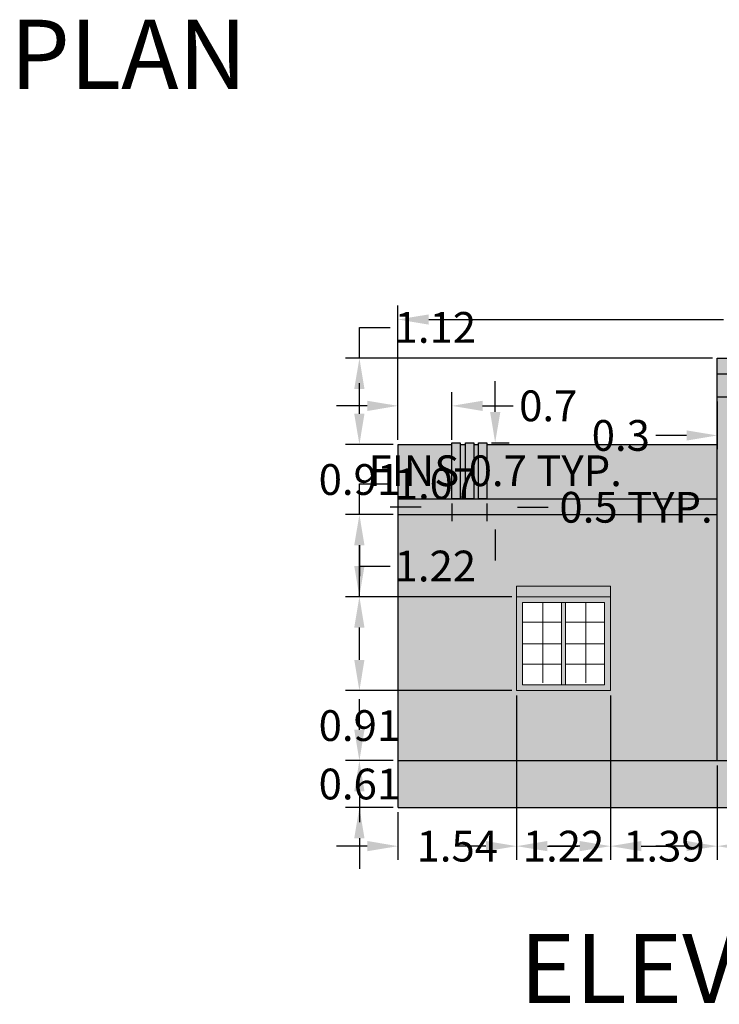
# Model space of a CAD drawing. Units: metres. Extents: x 24.2 to 58.5, y -14.5 to 15.2.
# Tile 1 of 7: x 29.8 to 38.9, y -14.5 to -1.7. Entities that reach past the tile are written whole.
import ezdxf

# ---------------------------------------------------------------- set-up
doc = ezdxf.new("R2010")
doc.units = ezdxf.units.M
doc.header["$MEASUREMENT"] = 0
for name, color, linetype, lineweight in [('A-ANNO-TITL', 1, 'Continuous', 30), ('A-ELEV', 7, 'Continuous', 25), ('A-ELEV-PATT', 61, 'Continuous', 13), ('A-GLAZ', 15, 'Continuous', 18), ('DIMENSION', 90, 'Continuous', 18)]:
    doc.layers.add(name, color=color, linetype=linetype, lineweight=lineweight)
doc.layers.add('A-ELEV-TRIM-PATT', color=251, linetype='Continuous', lineweight=13, true_color=0x636466)
doc.styles.get("Standard").update_dxf_attribs({"font": 'arial.ttf'})
doc.dimstyles.get("Standard").update_dxf_attribs({"dimtxt": 0.4, "dimasz": 0.4, "dimexe": 0.18, "dimexo": 0.0625, "dimgap": 0.09, "dimtad": 0, "dimtih": 1, "dimtoh": 1, "dimdec": 1, "dimzin": 0, "dimdsep": 46, "dimtxsty": 'Standard', "dimcen": 0.09, "dimadec": 0, "dimazin": 0, "dimtfac": 1, "dimtdec": 1, "dimtofl": 0, "dimtmove": 0, "dimatfit": 3, "dimfxl": 1, "dimtolj": 1, "dimtzin": 0, "dimarcsym": 0})

# ---------------------------------------------------------------- blocks, each defined once
blk = doc.blocks.new('PARAPET-TRIPLE-FIN')
for p, q in [((0.11, 0.707), (0.177, 0.707)), ((0.286, 0.707), (0.345, 0.707))]:
    blk.add_line(p, q)
for points in [[(0, 0.731), (0.11, 0.731), (0.11, 0), (0, 0)], [(0, 0.731), (0.11, 0.731), (0.11, 0), (0, 0)], [(0.177, 0.731), (0.286, 0.731), (0.286, 0), (0.177, 0)], [(0.345, 0.731), (0.455, 0.731), (0.455, 0), (0.345, 0)]]:
    blk.add_lwpolyline(points, close=True)
blk = doc.blocks.new('*D67')
at = {"layer": 'Defpoints', "color": 0, "transparency": 16777216}
for p in [(35.829, -7.164), (35.938, -7.164), (35.829, -7.895)]:
    blk.add_point(p, dxfattribs=at)
at = {"layer": 'DIMENSION', "color": 0, "lineweight": -2, "transparency": 16777216}
for p, q in [((35.938, -6.764), (35.938, -6.364)), ((35.891, -7.164), (36.118, -7.164)), ((35.891, -7.895), (36.118, -7.895)), ((35.938, -8.295), (35.938, -8.695))]:
    blk.add_line(p, q, dxfattribs=at)
at = {"layer": 'DIMENSION', "color": 0, "transparency": 16777216}
for points in [[(35.872, -6.764), (36.005, -6.764), (35.938, -7.164)], [(35.872, -8.295), (36.005, -8.295), (35.938, -7.895)]]:
    blk.add_solid(points, dxfattribs=at)
at = {"layer": 'DIMENSION', "color": 0, "transparency": 16777216, "insert": (35.938, -7.529), "char_height": 0.4, "attachment_point": 5}
blk.add_mtext('\\A1;FINS 0.7 TYP.', dxfattribs=at)
blk = doc.blocks.new('*D68')
at = {"layer": 'Defpoints', "color": 0, "transparency": 16777216}
for p in [(35.374, -7.895), (35.829, -7.895), (35.829, -8.004)]:
    blk.add_point(p, dxfattribs=at)
at = {"layer": 'DIMENSION', "color": 0, "lineweight": -2, "transparency": 16777216}
for p, q in [((34.974, -8.004), (34.574, -8.004)), ((35.374, -7.957), (35.374, -8.184)), ((35.829, -7.957), (35.829, -8.184)), ((36.229, -8.004), (36.629, -8.004))]:
    blk.add_line(p, q, dxfattribs=at)
at = {"layer": 'DIMENSION', "color": 0, "transparency": 16777216}
for points in [[(34.974, -7.938), (34.974, -8.071), (35.374, -8.004)], [(36.229, -7.938), (36.229, -8.071), (35.829, -8.004)]]:
    blk.add_solid(points, dxfattribs=at)
at = {"layer": 'DIMENSION', "color": 0, "transparency": 16777216, "insert": (37.77, -8.004), "char_height": 0.4, "attachment_point": 5}
blk.add_mtext('\\A1;0.5 TYP.', dxfattribs=at)
blk = doc.blocks.new('*D81')
at = {"layer": 'Defpoints', "color": 0, "transparency": 16777216}
for p in [(44.284, -5.562), (34.674, -7.188), (44.284, -7.188)]:
    blk.add_point(p, dxfattribs=at)
at = {"layer": 'DIMENSION', "color": 0, "lineweight": -2, "transparency": 16777216}
for p, q in [((34.674, -7.125), (34.674, -5.382)), ((44.284, -7.125), (44.284, -5.382)), ((35.074, -5.562), (38.908, -5.562)), ((43.884, -5.562), (40.05, -5.562))]:
    blk.add_line(p, q, dxfattribs=at)
at = {"layer": 'DIMENSION', "color": 0, "transparency": 16777216}
for points in [[(35.074, -5.496), (35.074, -5.629), (34.674, -5.562)], [(43.884, -5.496), (43.884, -5.629), (44.284, -5.562)]]:
    blk.add_solid(points, dxfattribs=at)
at = {"layer": 'DIMENSION', "color": 0, "transparency": 16777216, "insert": (39.479, -5.562), "char_height": 0.4, "attachment_point": 5}
blk.add_mtext('\\A1;9.61', dxfattribs=at)
blk = doc.blocks.new('*D83')
at = {"layer": 'Defpoints', "color": 0, "transparency": 16777216}
for p in [(34.172, -11.298), (34.674, -11.298), (34.674, -11.908)]:
    blk.add_point(p, dxfattribs=at)
at = {"layer": 'DIMENSION', "color": 0, "lineweight": -2, "transparency": 16777216}
for p, q in [((34.172, -10.898), (34.172, -10.498)), ((34.612, -11.298), (33.992, -11.298)), ((34.612, -11.908), (33.992, -11.908)), ((34.172, -12.308), (34.172, -12.708))]:
    blk.add_line(p, q, dxfattribs=at)
at = {"layer": 'DIMENSION', "color": 0, "transparency": 16777216}
for points in [[(34.105, -10.898), (34.238, -10.898), (34.172, -11.298)], [(34.105, -12.308), (34.238, -12.308), (34.172, -11.908)]]:
    blk.add_solid(points, dxfattribs=at)
at = {"layer": 'DIMENSION', "color": 0, "transparency": 16777216, "insert": (34.172, -11.603), "char_height": 0.4, "attachment_point": 5}
blk.add_mtext('\\A1;0.61', dxfattribs=at)
blk = doc.blocks.new('*D84')
at = {"layer": 'Defpoints', "color": 0, "transparency": 16777216}
for p in [(34.172, -10.388), (36.217, -10.388), (34.674, -11.298)]:
    blk.add_point(p, dxfattribs=at)
at = {"layer": 'DIMENSION', "color": 0, "lineweight": -2, "transparency": 16777216}
for p, q in [((34.172, -9.988), (34.172, -9.588)), ((36.154, -10.388), (33.992, -10.388)), ((34.612, -11.298), (33.992, -11.298)), ((34.172, -11.698), (34.172, -12.098))]:
    blk.add_line(p, q, dxfattribs=at)
at = {"layer": 'DIMENSION', "color": 0, "transparency": 16777216}
for points in [[(34.105, -9.988), (34.238, -9.988), (34.172, -10.388)], [(34.105, -11.698), (34.238, -11.698), (34.172, -11.298)]]:
    blk.add_solid(points, dxfattribs=at)
at = {"layer": 'DIMENSION', "color": 0, "transparency": 16777216, "insert": (34.172, -10.843), "char_height": 0.4, "attachment_point": 5}
blk.add_mtext('\\A1;0.91', dxfattribs=at)
blk = doc.blocks.new('*D85')
at = {"layer": 'Defpoints', "color": 0, "transparency": 16777216}
for p in [(34.172, -9.168), (36.217, -9.168), (36.217, -10.388)]:
    blk.add_point(p, dxfattribs=at)
at = {"layer": 'DIMENSION', "color": 0, "lineweight": -2, "transparency": 16777216}
for p, q in [((34.172, -9.168), (34.172, -8.768)), ((34.172, -8.768), (34.572, -8.768)), ((36.154, -9.168), (33.992, -9.168)), ((34.172, -9.988), (34.172, -9.568)), ((36.154, -10.388), (33.992, -10.388))]:
    blk.add_line(p, q, dxfattribs=at)
at = {"layer": 'DIMENSION', "color": 0, "transparency": 16777216}
for points in [[(34.105, -9.568), (34.238, -9.568), (34.172, -9.168)], [(34.105, -9.988), (34.238, -9.988), (34.172, -10.388)]]:
    blk.add_solid(points, dxfattribs=at)
at = {"layer": 'DIMENSION', "color": 0, "transparency": 16777216, "insert": (35.16, -8.768), "char_height": 0.4, "attachment_point": 5}
blk.add_mtext('\\A1;1.22', dxfattribs=at)
blk = doc.blocks.new('*D86')
at = {"layer": 'Defpoints', "color": 0, "transparency": 16777216}
for p in [(34.172, -8.098), (34.674, -8.098), (36.217, -9.168)]:
    blk.add_point(p, dxfattribs=at)
at = {"layer": 'DIMENSION', "color": 0, "lineweight": -2, "transparency": 16777216}
for p, q in [((34.172, -8.098), (34.172, -7.698)), ((34.172, -7.698), (34.572, -7.698)), ((34.612, -8.098), (33.992, -8.098)), ((34.172, -8.768), (34.172, -8.498)), ((36.154, -9.168), (33.992, -9.168))]:
    blk.add_line(p, q, dxfattribs=at)
at = {"layer": 'DIMENSION', "color": 0, "transparency": 16777216}
for points in [[(34.105, -8.498), (34.238, -8.498), (34.172, -8.098)], [(34.105, -8.768), (34.238, -8.768), (34.172, -9.168)]]:
    blk.add_solid(points, dxfattribs=at)
at = {"layer": 'DIMENSION', "color": 0, "transparency": 16777216, "insert": (35.162, -7.698), "char_height": 0.4, "attachment_point": 5}
blk.add_mtext('\\A1;1.07', dxfattribs=at)
blk = doc.blocks.new('*D87')
at = {"layer": 'Defpoints', "color": 0, "transparency": 16777216}
for p in [(34.172, -7.188), (34.674, -7.188), (34.674, -8.098)]:
    blk.add_point(p, dxfattribs=at)
at = {"layer": 'DIMENSION', "color": 0, "lineweight": -2, "transparency": 16777216}
for p, q in [((34.172, -6.788), (34.172, -6.388)), ((34.612, -7.188), (33.992, -7.188)), ((34.612, -8.098), (33.992, -8.098)), ((34.172, -8.498), (34.172, -8.898))]:
    blk.add_line(p, q, dxfattribs=at)
at = {"layer": 'DIMENSION', "color": 0, "transparency": 16777216}
for points in [[(34.105, -6.788), (34.238, -6.788), (34.172, -7.188)], [(34.105, -8.498), (34.238, -8.498), (34.172, -8.098)]]:
    blk.add_solid(points, dxfattribs=at)
at = {"layer": 'DIMENSION', "color": 0, "transparency": 16777216, "insert": (34.172, -7.643), "char_height": 0.4, "attachment_point": 5}
blk.add_mtext('\\A1;0.91', dxfattribs=at)
blk = doc.blocks.new('*D88')
at = {"layer": 'Defpoints', "color": 0, "transparency": 16777216}
for p in [(34.172, -6.065), (38.827, -6.065), (34.674, -7.188)]:
    blk.add_point(p, dxfattribs=at)
at = {"layer": 'DIMENSION', "color": 0, "lineweight": -2, "transparency": 16777216}
for p, q in [((34.172, -6.065), (34.172, -5.665)), ((34.172, -5.665), (34.572, -5.665)), ((38.764, -6.065), (33.992, -6.065)), ((34.172, -6.788), (34.172, -6.465)), ((34.612, -7.188), (33.992, -7.188))]:
    blk.add_line(p, q, dxfattribs=at)
at = {"layer": 'DIMENSION', "color": 0, "transparency": 16777216}
for points in [[(34.105, -6.465), (34.238, -6.465), (34.172, -6.065)], [(34.105, -6.788), (34.238, -6.788), (34.172, -7.188)]]:
    blk.add_solid(points, dxfattribs=at)
at = {"layer": 'DIMENSION', "color": 0, "transparency": 16777216, "insert": (35.16, -5.665), "char_height": 0.4, "attachment_point": 5}
blk.add_mtext('\\A1;1.12', dxfattribs=at)
blk = doc.blocks.new('*D90')
at = {"layer": 'Defpoints', "color": 0, "transparency": 16777216}
for p in [(36.217, -10.388), (34.674, -11.908), (36.217, -12.411)]:
    blk.add_point(p, dxfattribs=at)
at = {"layer": 'DIMENSION', "color": 0, "lineweight": -2, "transparency": 16777216}
for p, q in [((36.217, -10.451), (36.217, -12.591)), ((34.674, -11.971), (34.674, -12.591)), ((34.274, -12.411), (33.874, -12.411)), ((36.617, -12.411), (37.017, -12.411))]:
    blk.add_line(p, q, dxfattribs=at)
at = {"layer": 'DIMENSION', "color": 0, "transparency": 16777216}
for points in [[(34.274, -12.344), (34.274, -12.477), (34.674, -12.411)], [(36.617, -12.344), (36.617, -12.477), (36.217, -12.411)]]:
    blk.add_solid(points, dxfattribs=at)
at = {"layer": 'DIMENSION', "color": 0, "transparency": 16777216, "insert": (35.445, -12.411), "char_height": 0.4, "attachment_point": 5}
blk.add_mtext('\\A1;1.54', dxfattribs=at)
blk = doc.blocks.new('*D91')
at = {"layer": 'Defpoints', "color": 0, "transparency": 16777216}
for p in [(36.217, -10.388), (37.437, -10.388), (37.437, -12.411)]:
    blk.add_point(p, dxfattribs=at)
at = {"layer": 'DIMENSION', "color": 0, "lineweight": -2, "transparency": 16777216}
for p, q in [((36.217, -10.451), (36.217, -12.591)), ((37.437, -10.451), (37.437, -12.591)), ((35.817, -12.411), (35.417, -12.411)), ((37.837, -12.411), (38.237, -12.411))]:
    blk.add_line(p, q, dxfattribs=at)
at = {"layer": 'DIMENSION', "color": 0, "transparency": 16777216}
for points in [[(35.817, -12.344), (35.817, -12.477), (36.217, -12.411)], [(37.837, -12.344), (37.837, -12.477), (37.437, -12.411)]]:
    blk.add_solid(points, dxfattribs=at)
at = {"layer": 'DIMENSION', "color": 0, "transparency": 16777216, "insert": (36.827, -12.411), "char_height": 0.4, "attachment_point": 5}
blk.add_mtext('\\A1;1.22', dxfattribs=at)
blk = doc.blocks.new('*D92')
at = {"layer": 'Defpoints', "color": 0, "transparency": 16777216}
for p in [(37.437, -10.388), (38.827, -11.298), (38.827, -12.411)]:
    blk.add_point(p, dxfattribs=at)
at = {"layer": 'DIMENSION', "color": 0, "lineweight": -2, "transparency": 16777216}
for p, q in [((37.437, -10.451), (37.437, -12.591)), ((38.827, -11.361), (38.827, -12.591)), ((37.037, -12.411), (36.637, -12.411)), ((39.227, -12.411), (39.627, -12.411))]:
    blk.add_line(p, q, dxfattribs=at)
at = {"layer": 'DIMENSION', "color": 0, "transparency": 16777216}
for points in [[(37.037, -12.344), (37.037, -12.477), (37.437, -12.411)], [(39.227, -12.344), (39.227, -12.477), (38.827, -12.411)]]:
    blk.add_solid(points, dxfattribs=at)
at = {"layer": 'DIMENSION', "color": 0, "transparency": 16777216, "insert": (38.132, -12.411), "char_height": 0.4, "attachment_point": 5}
blk.add_mtext('\\A1;1.39', dxfattribs=at)
blk = doc.blocks.new('*D93')
at = {"layer": 'Defpoints', "color": 0, "transparency": 16777216}
for p in [(38.827, -11.298), (41.131, -11.298), (41.131, -12.411)]:
    blk.add_point(p, dxfattribs=at)
at = {"layer": 'DIMENSION', "color": 0, "lineweight": -2, "transparency": 16777216}
for p, q in [((38.827, -11.361), (38.827, -12.591)), ((41.131, -11.361), (41.131, -12.591)), ((38.427, -12.411), (38.027, -12.411)), ((41.531, -12.411), (41.931, -12.411))]:
    blk.add_line(p, q, dxfattribs=at)
at = {"layer": 'DIMENSION', "color": 0, "transparency": 16777216}
for points in [[(38.427, -12.344), (38.427, -12.477), (38.827, -12.411)], [(41.531, -12.344), (41.531, -12.477), (41.131, -12.411)]]:
    blk.add_solid(points, dxfattribs=at)
at = {"layer": 'DIMENSION', "color": 0, "transparency": 16777216, "insert": (39.979, -12.411), "char_height": 0.4, "attachment_point": 5}
blk.add_mtext('\\A1;2.305', dxfattribs=at)
blk = doc.blocks.new('*D98')
at = {"layer": 'Defpoints', "color": 0, "transparency": 16777216}
for p in [(35.374, -6.685), (34.674, -7.188), (35.374, -7.188)]:
    blk.add_point(p, dxfattribs=at)
at = {"layer": 'DIMENSION', "color": 0, "lineweight": -2, "transparency": 16777216}
for p, q in [((34.674, -7.125), (34.674, -6.505)), ((35.374, -7.125), (35.374, -6.505)), ((34.274, -6.685), (33.874, -6.685)), ((35.774, -6.685), (36.174, -6.685))]:
    blk.add_line(p, q, dxfattribs=at)
at = {"layer": 'DIMENSION', "color": 0, "transparency": 16777216}
for points in [[(34.274, -6.619), (34.274, -6.752), (34.674, -6.685)], [(35.774, -6.619), (35.774, -6.752), (35.374, -6.685)]]:
    blk.add_solid(points, dxfattribs=at)
at = {"layer": 'DIMENSION', "color": 0, "transparency": 16777216, "insert": (36.628, -6.685), "char_height": 0.4, "attachment_point": 5}
blk.add_mtext('\\A1;0.7', dxfattribs=at)
blk = doc.blocks.new('*D102')
at = {"layer": 'Defpoints', "color": 0, "transparency": 16777216}
for p in [(38.827, -6.568), (39.127, -6.568), (38.827, -7.07)]:
    blk.add_point(p, dxfattribs=at)
at = {"layer": 'DIMENSION', "color": 0, "lineweight": -2, "transparency": 16777216}
for p, q in [((38.827, -6.63), (38.827, -7.25)), ((39.127, -6.63), (39.127, -7.25)), ((38.427, -7.07), (38.027, -7.07)), ((39.527, -7.07), (39.927, -7.07))]:
    blk.add_line(p, q, dxfattribs=at)
at = {"layer": 'DIMENSION', "color": 0, "transparency": 16777216}
for points in [[(38.427, -7.004), (38.427, -7.137), (38.827, -7.07)], [(39.527, -7.004), (39.527, -7.137), (39.127, -7.07)]]:
    blk.add_solid(points, dxfattribs=at)
at = {"layer": 'DIMENSION', "color": 0, "transparency": 16777216, "insert": (37.572, -7.07), "char_height": 0.4, "attachment_point": 5}
blk.add_mtext('\\A1;0.3', dxfattribs=at)

msp = doc.modelspace()

# ---------------------------------------------------------------- hatches: boundary and pattern name
at = {"layer": 'A-ELEV-PATT', "transparency": 33554567}
h = msp.add_hatch(color=256, dxfattribs=at)
h.dxf.hatch_style = 1
h.paths.add_polyline_path([(38.8266, -8.0979), (34.6742, -8.0979), (34.6742, -11.2983), (38.8266, -11.2983)])
h.paths.add_polyline_path([(37.4366, -10.3883), (36.2166, -10.3883), (36.2166, -9.1683), (36.2166, -9.0299), (37.4366, -9.0299), (37.4366, -9.1683)], flags=16)
h.paths.add_polyline_path([(37.3604, -10.3121), (36.2928, -10.3121), (36.2928, -9.2445), (36.8012, -9.2445), (37.3604, -9.2445)], flags=0)
h.paths.add_polyline_path([(37.1162, -10.0461), (36.852, -10.0461), (36.852, -9.2445), (37.1162, -9.2445)], flags=0)
h.paths.add_polyline_path([(36.8012, -10.0461), (36.557, -10.0461), (36.557, -9.4996), (36.8012, -9.4996)], flags=0)
h.paths.add_polyline_path([(44.2838, -8.0979), (41.1314, -8.0979), (41.1314, -11.2983), (41.3209, -11.2983), (41.3209, -9.1643), (42.2309, -9.1643), (42.2309, -11.2983), (44.2838, -11.2983)])
h.paths.add_polyline_path([(42.8811, -9.0437), (43.4811, -9.0437), (43.4811, -9.1643), (43.4811, -10.0743), (42.8811, -10.0743), (42.8811, -9.1643)], flags=16)
h.paths.add_polyline_path([(42.9573, -9.2405), (43.4049, -9.2405), (43.4049, -9.9981), (42.9573, -9.9981)], flags=0)
h.paths.add_polyline_path([(44.2838, -7.8947), (41.1314, -7.8947), (41.1314, -8.0979), (44.2838, -8.0979)])
h.paths.add_polyline_path([(38.8266, -7.8947), (34.6742, -7.8947), (34.6742, -8.0979), (38.8266, -8.0979)])
h.paths.add_polyline_path([(41.1314, -6.2679), (38.8266, -6.2679), (38.8266, -6.5679), (41.1314, -6.5679)])
h.paths.add_polyline_path([(39.1266, -6.5679), (38.8266, -6.5679), (38.8266, -11.2983), (39.1266, -11.2983)])
h.paths.add_polyline_path([(41.1314, -6.5679), (40.8314, -6.5679), (40.8314, -11.2983), (41.1314, -11.2983), (41.1314, -8.0979)])
h.paths.add_polyline_path([(35.4837, -7.1642), (35.3742, -7.1642), (35.3742, -7.8947), (35.4837, -7.8947)])
h.paths.add_polyline_path([(35.6603, -7.1642), (35.5509, -7.1642), (35.5509, -7.8947), (35.6603, -7.8947)])
h.paths.add_polyline_path([(35.8286, -7.1642), (35.7192, -7.1642), (35.7192, -7.8947), (35.8286, -7.8947)])
h.paths.add_polyline_path([(43.3078, -7.1642), (43.1983, -7.1642), (43.1983, -7.8947), (43.3078, -7.8947)])
h.paths.add_polyline_path([(43.4844, -7.1642), (43.3749, -7.1642), (43.3749, -7.8947), (43.4844, -7.8947)])
h.paths.add_polyline_path([(43.6527, -7.1642), (43.5433, -7.1642), (43.5433, -7.8947), (43.6527, -7.8947)])
at = {"layer": 'A-ELEV-TRIM-PATT', "transparency": 33554567}
h = msp.add_hatch(color=256, dxfattribs=at)
h.dxf.hatch_style = 1
h.paths.add_polyline_path([(40.8314, -6.5679), (39.1266, -6.5679), (39.1266, -11.2983), (40.8314, -11.2983)])
h.paths.add_polyline_path([(44.2838, -11.2983), (34.6742, -11.2983), (34.6742, -11.9083), (44.2838, -11.9083)])
h.paths.add_polyline_path([(38.8266, -7.1879), (35.8286, -7.1879), (35.8286, -7.8947), (38.8266, -7.8947)])
h.paths.add_polyline_path([(35.3742, -7.1879), (34.6742, -7.1879), (34.6742, -7.8947), (35.3742, -7.8947)])
h.paths.add_polyline_path([(35.5509, -7.1879), (35.4837, -7.1879), (35.4837, -7.8947), (35.5509, -7.8947)])
h.paths.add_polyline_path([(35.7192, -7.1879), (35.6603, -7.1879), (35.6603, -7.8947), (35.7192, -7.8947)])
h.paths.add_polyline_path([(43.1983, -7.1879), (41.1314, -7.1879), (41.1314, -7.8947), (43.1983, -7.8947)])
h.paths.add_polyline_path([(44.2838, -7.1879), (43.6527, -7.1879), (43.6527, -7.8947), (44.2838, -7.8947)])
h.paths.add_polyline_path([(43.3749, -7.1879), (43.3078, -7.1879), (43.3078, -7.8947), (43.3749, -7.8947)])
h.paths.add_polyline_path([(43.5433, -7.1879), (43.4844, -7.1879), (43.4844, -7.8947), (43.5433, -7.8947)])
h.paths.add_polyline_path([(41.1314, -6.0647), (38.8266, -6.0647), (38.8266, -6.2679), (41.1314, -6.2679)])
h = msp.add_hatch(color=256, dxfattribs=at)
h.dxf.hatch_style = 1
h.paths.add_polyline_path([(37.4366, -9.1683), (37.4366, -9.0299), (36.2166, -9.0299), (36.2166, -9.1683)])
h.paths.add_polyline_path([(42.8811, -9.0437), (42.8811, -9.1643), (43.4811, -9.1643), (43.4811, -9.0437)])
h = msp.add_hatch(color=256, dxfattribs=at)
h.dxf.hatch_style = 1
h.paths.add_polyline_path([(36.2166, -10.3883), (37.4366, -10.3883), (37.4366, -9.1683), (36.2166, -9.1683)])
h.paths.add_polyline_path([(36.2928, -9.2445), (37.3604, -9.2445), (37.3604, -10.3121), (36.2928, -10.3121)], flags=16)
h.paths.add_polyline_path([(43.4811, -9.1643), (42.8811, -9.1643), (42.8811, -10.0743), (43.4811, -10.0743)])
h.paths.add_polyline_path([(43.4049, -9.9981), (42.9573, -9.9981), (42.9573, -9.2405), (43.4049, -9.2405)], flags=16)
h = msp.add_hatch(color=256, dxfattribs=at)
h.dxf.hatch_style = 1
h.paths.add_polyline_path([(36.852, -9.2445), (36.8012, -9.2445), (36.8012, -10.3121), (36.852, -10.3121)])

# ---------------------------------------------------------------- linework, layer by layer
at = {"layer": 'A-ELEV'}
for p, q in [((38.8266, -11.2983), (38.8266, -6.0647)), ((38.8266, -6.0647), (41.1314, -6.0647)), ((38.8266, -6.2679), (41.1314, -6.2679)), ((38.8266, -6.5679), (41.1314, -6.5679)), ((34.6742, -11.9083), (34.6742, -7.1879)), ((34.6742, -7.1879), (35.3742, -7.1879)), ((35.8286, -7.1879), (38.8266, -7.1879)), ((34.6742, -7.8947), (38.8266, -7.8947)), ((34.6742, -8.0979), (38.8266, -8.0979)), ((34.6742, -11.2983), (44.2838, -11.2983)), ((34.6742, -11.9083), (44.2838, -11.9083))]:
    msp.add_line(p, q, dxfattribs=at)
at = {"layer": 'A-GLAZ'}
for p, q in [((37.4366, -9.1683), (36.2166, -9.1683)), ((36.2166, -9.1683), (36.2166, -10.3883)), ((37.4366, -10.3883), (37.4366, -9.1683)), ((37.3604, -9.2445), (36.2928, -9.2445)), ((36.2928, -9.2445), (36.2928, -10.3121)), ((36.2928, -9.2445), (36.8012, -9.2445)), ((36.557, -9.2445), (36.557, -10.2879)), ((36.8012, -10.3121), (36.8012, -9.2445)), ((36.852, -10.3121), (36.852, -9.2445)), ((36.852, -9.2445), (37.3604, -9.2445)), ((37.1162, -9.2445), (37.1162, -10.2879)), ((37.3604, -10.3121), (37.3604, -9.2445)), ((36.8012, -9.4996), (36.2928, -9.4996)), ((37.3604, -9.4996), (36.852, -9.4996)), ((36.8012, -9.7783), (36.2928, -9.7783)), ((37.3604, -9.7783), (36.852, -9.7783)), ((36.8012, -10.0461), (36.2928, -10.0461)), ((37.3604, -10.0461), (36.852, -10.0461)), ((36.2928, -10.3121), (37.3604, -10.3121)), ((36.2166, -10.3883), (37.4366, -10.3883))]:
    msp.add_line(p, q, dxfattribs=at)
msp.add_lwpolyline([(36.2166, -9.1683), (37.4366, -9.1683), (37.4366, -9.0299), (36.2166, -9.0299)], close=True, dxfattribs=at)

# ---------------------------------------------------------------- block references
at = {"layer": 'A-ELEV'}
msp.add_blockref('PARAPET-TRIPLE-FIN', (35.374, -7.895), dxfattribs=at)

# ---------------------------------------------------------------- texts
at = {"layer": 'A-ANNO-TITL', "char_height": 0.9, "attachment_point": 2}
for s, insert in [('PLAN', (31.1687, -1.6633)), ('ELEVATION', (39.4872, -13.5517))]:
    msp.add_mtext_dynamic_manual_height_columns(s, width=1.744906, gutter_width=1, heights=[0], dxfattribs=dict(at, insert=insert))

# ---------------------------------------------------------------- dimensions: what is measured, and where the dimension line sits
at = {"layer": 'DIMENSION'}
for base, p1, p2, override, picture, middle in [((44.2838, -5.5622), (34.6742, -7.1879), (44.2838, -7.1879), {"dimdec": 2, "dimlfac": 1, "dimrnd": 0, "dimzin": 0, "dimdsep": 46, "dimlunit": 2}, '*D81', (39.479, -5.5622)), ((35.3742, -6.6854), (34.6742, -7.1879), (35.3742, -7.1879), {"dimdec": 1, "dimlfac": 1, "dimrnd": 0, "dimzin": 0, "dimdsep": 46, "dimlunit": 2}, '*D98', (36.6284, -6.6854)), ((36.2166, -12.4108), (34.6742, -11.9083), (36.2166, -10.3883), {"dimdec": 2, "dimlfac": 1, "dimrnd": 0, "dimzin": 0, "dimdsep": 46, "dimlunit": 2}, '*D90', (35.4454, -12.4108)), ((37.4366, -12.4108), (36.2166, -10.3883), (37.4366, -10.3883), {"dimdec": 2, "dimlfac": 1, "dimrnd": 0, "dimzin": 0, "dimdsep": 46, "dimlunit": 2}, '*D91', (36.8266, -12.4108)), ((38.8266, -12.4108), (37.4366, -10.3883), (38.8266, -11.2983), {"dimdec": 2, "dimlfac": 1, "dimrnd": 0, "dimzin": 0, "dimdsep": 46, "dimlunit": 2}, '*D92', (38.1316, -12.4108)), ((41.1314, -12.4108), (38.8266, -11.2983), (41.1314, -11.2983), {"dimdec": 3, "dimlfac": 1, "dimrnd": 0, "dimzin": 0, "dimdsep": 46, "dimlunit": 2}, '*D93', (39.979, -12.4108))]:
    dim = msp.add_linear_dim(base=base, p1=p1, p2=p2, dimstyle='Standard', override=override, dxfattribs=at)
    dim.commit()
    dim.dimension.update_dxf_attribs({"geometry": picture, "text_midpoint": middle})
for base, p1, p2, angle, override, picture, middle in [((34.1717, -6.0647), (34.6742, -7.1879), (38.8266, -6.0647), 90, {"dimdec": 2, "dimlfac": 1, "dimrnd": 0, "dimzin": 0, "dimdsep": 46, "dimlunit": 2}, '*D88', (35.1603, -5.6647)), ((34.1717, -7.1879), (34.6742, -8.0979), (34.6742, -7.1879), 90, {"dimdec": 2, "dimlfac": 1, "dimrnd": 0, "dimzin": 0, "dimdsep": 46, "dimlunit": 2}, '*D87', (34.1717, -7.6429)), ((38.8266, -7.0704), (39.1266, -6.5679), (38.8266, -6.5679), 180, {"dimdec": 1, "dimlfac": 1, "dimrnd": 0, "dimzin": 0, "dimdsep": 46, "dimlunit": 2}, '*D102', (37.5725, -7.0704)), ((34.1717, -8.0979), (36.2166, -9.1683), (34.6742, -8.0979), 90, {"dimdec": 2, "dimlfac": 1, "dimrnd": 0, "dimzin": 0, "dimdsep": 46, "dimlunit": 2}, '*D86', (35.1624, -7.6979)), ((34.1717, -9.1683), (36.2166, -10.3883), (36.2166, -9.1683), 90, {"dimdec": 2, "dimlfac": 1, "dimrnd": 0, "dimzin": 0, "dimdsep": 46, "dimlunit": 2}, '*D85', (35.1603, -8.7683)), ((34.1717, -10.3883), (34.6742, -11.2983), (36.2166, -10.3883), 90, {"dimdec": 2, "dimlfac": 1, "dimrnd": 0, "dimzin": 0, "dimdsep": 46, "dimlunit": 2}, '*D84', (34.1717, -10.8433)), ((34.1717, -11.2983), (34.6742, -11.9083), (34.6742, -11.2983), 90, {"dimdec": 2, "dimlfac": 1, "dimrnd": 0, "dimzin": 0, "dimdsep": 46, "dimlunit": 2}, '*D83', (34.1717, -11.6033))]:
    dim = msp.add_linear_dim(base=base, p1=p1, p2=p2, angle=angle, dimstyle='Standard', override=override, dxfattribs=at)
    dim.commit()
    dim.dimension.update_dxf_attribs({"geometry": picture, "text_midpoint": middle})
dim = msp.add_linear_dim(base=(35.9382, -7.1642), p1=(35.8286, -7.8947), p2=(35.8286, -7.1642), angle=90, text='FINS <> TYP.', dimstyle='Standard', override={"dimdec": 1, "dimlfac": 1, "dimrnd": 0, "dimzin": 0, "dimdsep": 46, "dimlunit": 2}, dxfattribs=at)
dim.commit()
dim.dimension.update_dxf_attribs({"geometry": '*D67', "text_midpoint": (35.9382, -7.5295)})
dim = msp.add_linear_dim(base=(35.8286, -8.0043), p1=(35.3742, -7.8947), p2=(35.8286, -7.8947), text='<> TYP.', dimstyle='Standard', override={"dimdec": 1, "dimlfac": 1, "dimrnd": 0, "dimzin": 0, "dimdsep": 46, "dimlunit": 2}, dxfattribs=at)
dim.commit()
dim.dimension.update_dxf_attribs({"geometry": '*D68', "text_midpoint": (37.7698, -8.0043)})

doc.saveas('drawing.dxf')
